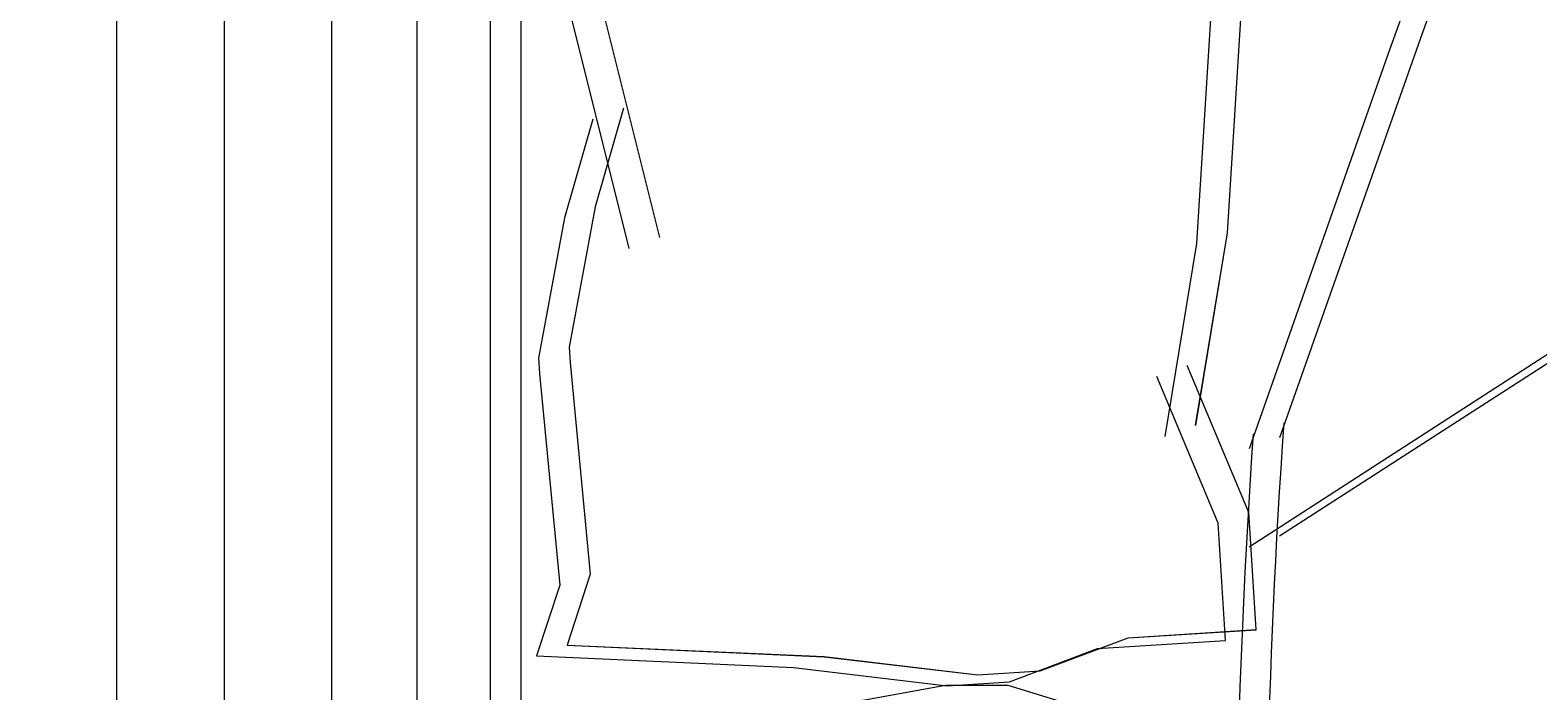
# Model space of a CAD drawing. Units: inches. Extents: x 1885 to 2748, y 783 to 2421.
# Tile 9 of 117: x 1969 to 2001, y 1164 to 1178. Entities that reach past the tile are written whole.
import ezdxf

# ---------------------------------------------------------------- set-up
doc = ezdxf.new("R2010")
doc.units = ezdxf.units.IN
for name, color, linetype, lineweight in [('A-ANNO-DIMS', 2, 'Continuous', 18), ('A-FURN', 8, 'Continuous', 13), ('A-GLAZ', 181, 'Continuous', 18)]:
    doc.layers.add(name, color=color, linetype=linetype, lineweight=lineweight)
doc.styles.get("Standard").update_dxf_attribs({"font": 'arial.ttf'})
doc.dimstyles.get("Standard").update_dxf_attribs({"dimtxt": 0.18, "dimasz": 0.18, "dimexe": 0.18, "dimexo": 0.0625, "dimgap": 0.09, "dimtad": 0, "dimtih": 1, "dimtoh": 1, "dimdec": 4, "dimzin": 0, "dimdsep": 46, "dimtxsty": 'Standard', "dimcen": 0.09, "dimadec": 0, "dimazin": 0, "dimtfac": 1, "dimtdec": 4, "dimtofl": 0, "dimtmove": 0, "dimatfit": 3, "dimfxl": 1, "dimtolj": 1, "dimtzin": 0, "dimarcsym": 0})

# ---------------------------------------------------------------- blocks, each defined once
blk = doc.blocks.new('BED-DOUBLE')
for p, q in [((0.004, 3.474), (0.004, 51.493)), ((2.177, 3.702), (2.177, 51.493)), ((2.177, 3.702), (2.177, 51.492)), ((1.537, 3.474), (1.537, 51.264)), ((1.537, 3.474), (1.537, 51.264)), ((22.972, 46.447), (20.96, 40.871)), ((22.972, 46.447), (20.96, 40.871)), ((22.332, 46.218), (20.32, 40.643)), ((22.332, 46.218), (20.32, 40.643)), ((16.938, 36.823), (17.369, 43.833)), ((16.938, 36.823), (17.369, 43.833)), ((16.299, 36.595), (16.73, 43.605)), ((16.299, 36.595), (16.73, 43.605)), ((3.073, 41.913), (4.426, 36.494)), ((3.073, 41.913), (4.426, 36.493)), ((3.712, 42.141), (5.065, 36.722)), ((3.712, 42.141), (5.065, 36.722)), ((20.32, 40.643), (17.387, 32.305)), ((20.32, 40.643), (17.387, 32.305)), ((20.96, 40.871), (18.026, 32.533)), ((20.96, 40.871), (18.026, 32.533)), ((4.317, 39.427), (3.721, 37.362)), ((4.317, 39.427), (3.721, 37.362)), ((3.677, 39.199), (3.082, 37.134)), ((3.677, 39.199), (3.082, 37.134)), ((3.721, 37.362), (3.18, 34.432)), ((3.721, 37.362), (3.18, 34.431)), ((3.082, 37.134), (2.541, 34.203)), ((3.082, 37.134), (2.541, 34.203)), ((15.632, 32.563), (16.299, 36.595)), ((15.632, 32.563), (16.299, 36.595)), ((16.271, 32.791), (16.938, 36.823)), ((16.272, 32.791), (16.938, 36.823)), ((18.026, 30.486), (24.519, 34.676)), ((18.026, 30.486), (24.519, 34.676)), ((3.18, 34.432), (3.2, 34.111)), ((3.18, 34.431), (3.2, 34.11)), ((17.387, 30.258), (23.88, 34.448)), ((17.387, 30.258), (23.88, 34.448)), ((2.541, 34.203), (2.561, 33.882)), ((2.541, 34.203), (2.561, 33.882)), ((3.2, 34.111), (3.622, 29.683)), ((3.2, 34.11), (3.622, 29.683)), ((17.382, 30.977), (16.097, 34.048)), ((17.382, 30.977), (16.097, 34.048)), ((2.561, 33.882), (2.982, 29.454)), ((2.561, 33.882), (2.982, 29.454)), ((16.743, 30.749), (15.458, 33.819)), ((16.743, 30.749), (15.458, 33.819)), ((17.536, 28.525), (17.382, 30.977)), ((17.536, 28.524), (17.382, 30.977)), ((16.896, 28.296), (16.743, 30.749)), ((16.896, 28.296), (16.743, 30.749)), ((3.622, 29.683), (3.135, 28.204)), ((3.622, 29.683), (3.135, 28.204)), ((2.982, 29.454), (2.495, 27.976)), ((2.982, 29.454), (2.495, 27.975)), ((13.02, 27.663), (14.86, 28.357)), ((13.02, 27.663), (14.86, 28.357)), ((14.86, 28.357), (17.536, 28.525)), ((14.86, 28.357), (17.536, 28.524)), ((3.135, 28.204), (8.51, 27.961)), ((3.135, 28.204), (8.51, 27.96)), ((12.38, 27.435), (14.22, 28.129)), ((12.38, 27.434), (14.22, 28.129)), ((14.22, 28.129), (16.896, 28.296)), ((14.22, 28.129), (16.896, 28.296)), ((2.495, 27.976), (7.871, 27.732)), ((2.495, 27.975), (7.871, 27.732)), ((7.871, 27.732), (11.082, 27.354)), ((7.871, 27.732), (11.082, 27.353)), ((8.51, 27.961), (11.721, 27.582)), ((8.51, 27.96), (11.721, 27.582)), ((11.082, 27.354), (12.38, 27.435)), ((11.082, 27.353), (12.38, 27.434)), ((11.721, 27.582), (13.02, 27.663)), ((11.721, 27.582), (13.02, 27.663)), ((7.863, 26.788), (11.044, 27.366)), ((7.863, 26.788), (11.044, 27.366)), ((11.044, 27.366), (12.345, 27.366)), ((11.044, 27.366), (12.345, 27.366)), ((12.345, 27.366), (14.225, 26.788)), ((12.345, 27.366), (14.225, 26.788))]:
    blk.add_line(p, q)
for centre in [(182.695, 21.586), (182.695, 21.586), (182.056, 21.358), (182.056, 21.357)]:
    blk.add_arc(centre, 164.969, 176.08655, 186.78213)
blk = doc.blocks.new('WIN-60')
for p, q in [((0.004, 59.998), (0.004, -0.002)), ((2.254, 59.998), (2.254, -0.002)), ((4.504, -0.002), (4.504, 59.998))]:
    blk.add_line(p, q)
blk = doc.blocks.new('*D45')
at = {"layer": 'A-ANNO-DIMS', "color": 0, "lineweight": -2, "transparency": 16777216}
for p, q in [((1980.711, 1524.006), (1902.844, 1524.006)), ((1903.024, 1523.826), (1903.024, 1290.937)), ((1903.024, 1057.686), (1903.024, 1290.574)), ((1971.211, 1057.506), (1902.844, 1057.506))]:
    blk.add_line(p, q, dxfattribs=at)
at = {"layer": 'A-ANNO-DIMS', "color": 0, "transparency": 16777216}
for points in [[(1902.994, 1523.826), (1903.054, 1523.826), (1903.024, 1524.006)], [(1902.994, 1057.686), (1903.054, 1057.686), (1903.024, 1057.506)]]:
    blk.add_solid(points, dxfattribs=at)
at = {"layer": 'Defpoints', "color": 0, "transparency": 16777216}
for p in [(1903.024, 1524.006), (1980.774, 1524.006), (1971.274, 1057.506)]:
    blk.add_point(p, dxfattribs=at)
at = {"layer": 'A-ANNO-DIMS', "color": 0, "transparency": 16777216, "insert": (1903.024, 1290.756), "char_height": 0.18, "attachment_point": 5}
blk.add_mtext('\\A1;466.5', dxfattribs=at)

msp = doc.modelspace()

# ---------------------------------------------------------------- block references
at = {"layer": 'A-FURN'}
msp.add_blockref('BED-DOUBLE', (1977.555, 1137.199), dxfattribs=at)
at = {"layer": 'A-GLAZ'}
msp.add_blockref('WIN-60', (1971.27, 1145.64), dxfattribs=at)

# ---------------------------------------------------------------- dimensions: what is measured, and where the dimension line sits
at = {"layer": 'A-ANNO-DIMS'}
dim = msp.add_linear_dim(base=(1903.024, 1524.006), p1=(1971.274, 1057.506), p2=(1980.774, 1524.006), angle=90, dimstyle='Standard', override={"dimdec": 1, "dimlfac": 1, "dimrnd": 0, "dimzin": 0, "dimdsep": 46, "dimlunit": 2}, dxfattribs=at)
dim.commit()
dim.dimension.update_dxf_attribs({"geometry": '*D45', "text_midpoint": (1903.024, 1290.756)})

doc.saveas('drawing.dxf')
